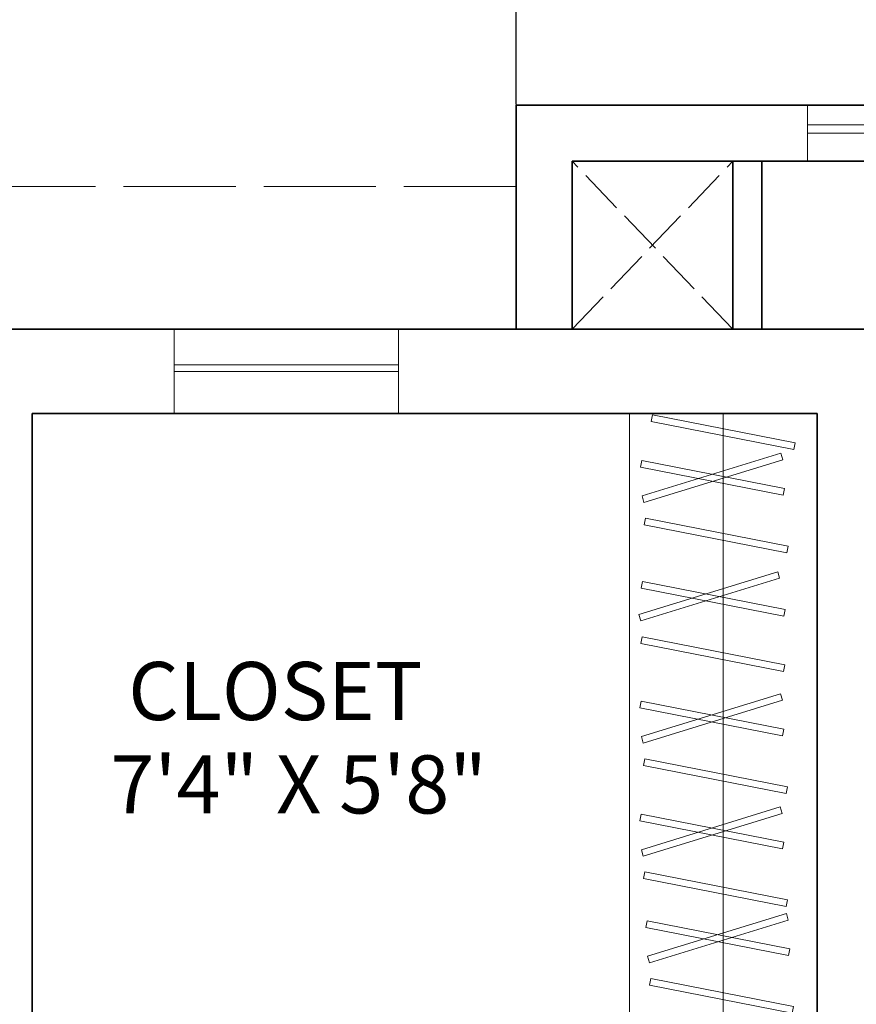
# Model space of a CAD drawing. Units: inches. Extents: x -61 to 1599, y -1316 to 257.
# Tile 172 of 204: x 1214 to 1304, y -684 to -579. Entities that reach past the tile are written whole.
import ezdxf

# ---------------------------------------------------------------- set-up
doc = ezdxf.new("R2010")
doc.units = ezdxf.units.IN
doc.header["$MEASUREMENT"] = 0
doc.linetypes.add('ACAD_ISO02W100', pattern=[15, 12, -3])
for name, color, linetype, lineweight in [('A-ANNO-DIMS', 2, 'Continuous', 18), ('A-AREA-IDEN', 1, 'Continuous', 18), ('A-FLOR-CASE', 8, 'Continuous', 18), ('A-FLOR-OPEN-HIDN', 8, 'ACAD_ISO02W100', 13), ('A-FLOR-OVHD', 203, 'ACAD_ISO02W100', 13), ('WALLS', 4, 'Continuous', 35), ('WINDOWS', 220, 'Continuous', 18)]:
    doc.layers.add(name, color=color, linetype=linetype, lineweight=lineweight)
doc.styles.get("Standard").update_dxf_attribs({"font": 'arial.ttf'})
doc.dimstyles.get("Standard").update_dxf_attribs({"dimtxt": 0.18, "dimasz": 0.18, "dimexe": 0.18, "dimexo": 0.0625, "dimgap": 0.09, "dimtad": 0, "dimtih": 1, "dimtoh": 1, "dimdec": 0, "dimzin": 0, "dimdsep": 46, "dimlunit": 3, "dimtxsty": 'Standard', "dimcen": 0.09, "dimadec": 0, "dimazin": 0, "dimtfac": 1, "dimtdec": 0, "dimtofl": 0, "dimtmove": 0, "dimatfit": 3, "dimfxl": 1, "dimtolj": 1, "dimtzin": 0, "dimarcsym": 0})

# ---------------------------------------------------------------- blocks, each defined once
blk = doc.blocks.new('WIN-24IN')
for p, q in [((0, 4.5), (0, 9)), ((0, 9), (0, 0)), ((24, 9), (24, 0)), ((0, 5.19), (24, 5.19)), ((0, 4.5), (24, 4.5))]:
    blk.add_line(p, q)
blk = doc.blocks.new('WIN-51IN')
for p, q in [((0, 0), (0, 6)), ((50.52, 0), (50.52, 6)), ((0, 3.89), (50.52, 3.89)), ((0, 3), (50.52, 3))]:
    blk.add_line(p, q)
blk = doc.blocks.new('WARDROBE-HANGING')
blk.add_line((10.05, 0), (10.05, 68))
for points in [[(20.09, 0), (0, 0), (0, 68), (20.09, 68)], [(2.48, 67.85), (17.75, 64.85), (17.61, 64.14), (2.34, 67.15)], [(1.35, 59.16), (16.22, 63.73), (16.43, 63.04), (1.56, 58.47)], [(1.32, 62.96), (16.59, 59.95), (16.45, 59.25), (1.19, 62.25)], [(1.71, 56.78), (16.98, 53.78), (16.84, 53.07), (1.57, 56.08)], [(1, 46.47), (15.87, 51.04), (16.08, 50.35), (1.21, 45.78)], [(1.39, 50.01), (16.66, 47.01), (16.52, 46.3), (1.26, 49.31)], [(1.36, 44.09), (16.63, 41.09), (16.49, 40.38), (1.23, 43.38)], [(1.28, 33.41), (16.16, 37.98), (16.37, 37.29), (1.49, 32.72)], [(1.26, 37.2), (16.53, 34.2), (16.39, 33.49), (1.12, 36.5)], [(1.65, 31.03), (16.92, 28.03), (16.78, 27.32), (1.51, 30.32)], [(1.28, 21.3), (16.15, 25.87), (16.36, 25.18), (1.49, 20.61)], [(1.26, 25.09), (16.53, 22.09), (16.39, 21.38), (1.12, 24.39)], [(1.65, 18.92), (16.91, 15.92), (16.78, 15.21), (1.51, 18.21)], [(1.93, 9.89), (16.8, 14.46), (17.01, 13.77), (2.14, 9.2)], [(1.91, 13.69), (17.17, 10.68), (17.04, 9.98), (1.77, 12.98)], [(2.29, 7.51), (17.56, 4.51), (17.42, 3.8), (2.16, 6.81)], [(17.49, 1.96), (1.93, 1.96), (1.93, 2.68), (17.49, 2.68)]]:
    blk.add_lwpolyline(points, close=True)
blk = doc.blocks.new('*D708')
at = {"layer": 'A-ANNO-DIMS', "color": 0, "lineweight": -2, "transparency": 16777216}
for p, q in [((1267.48, -588.11), (1267.48, 257.46)), ((1267.66, 257.28), (1324.14, 257.28)), ((1381.52, 257.28), (1325.05, 257.28)), ((1381.7, -588.11), (1381.7, 257.46))]:
    blk.add_line(p, q, dxfattribs=at)
at = {"layer": 'A-ANNO-DIMS', "color": 0, "transparency": 16777216}
for points in [[(1267.66, 257.31), (1267.66, 257.25), (1267.48, 257.28)], [(1381.52, 257.31), (1381.52, 257.25), (1381.7, 257.28)]]:
    blk.add_solid(points, dxfattribs=at)
at = {"layer": 'DEFPOINTS', "color": 0, "transparency": 16777216}
for p in [(1381.7, 257.28), (1267.48, -588.17), (1381.7, -588.17)]:
    blk.add_point(p, dxfattribs=at)
at = {"layer": 'A-ANNO-DIMS', "color": 0, "transparency": 16777216, "insert": (1324.59, 257.28), "char_height": 0.18, "attachment_point": 5}
blk.add_mtext('\\A1;114.22', dxfattribs=at)

msp = doc.modelspace()

# ---------------------------------------------------------------- linework, layer by layer
at = {"layer": 'A-FLOR-OPEN-HIDN', "ltscale": 0.4}
for p, q in [((1273.4807, -612.169), (1290.6819, -594.169)), ((1290.6819, -612.169), (1273.4807, -594.169))]:
    msp.add_line(p, q, dxfattribs=at)
at = {"layer": 'A-FLOR-OVHD'}
msp.add_line((1267.4807, -596.8766), (1138.8585, -596.8766), dxfattribs=at)
at = {"layer": 'WALLS'}
for p, q in [((1267.4807, -612.169), (1267.4807, -588.169)), ((1381.7028, -588.169), (1267.4807, -588.169)), ((1273.4807, -612.169), (1273.4807, -594.169)), ((1375.7028, -594.169), (1273.4807, -594.169)), ((1290.6819, -612.169), (1290.6819, -594.169)), ((1293.7747, -612.169), (1293.7747, -594.169)), ((1522.7028, -612.169), (992.7028, -612.169)), ((1215.7028, -621.169), (1215.7028, -689.169)), ((1215.7028, -621.169), (1299.7028, -621.169)), ((1299.7028, -621.169), (1299.7028, -689.169))]:
    msp.add_line(p, q, dxfattribs=at)

# ---------------------------------------------------------------- block references
at = {"layer": 'A-FLOR-CASE'}
msp.add_blockref('WARDROBE-HANGING', (1279.609, -689.1691), dxfattribs=at)
at = {"layer": 'WINDOWS'}
for name, p in [('WIN-51IN', (1298.659, -594.1691)), ('WIN-24IN', (1230.882, -621.1691))]:
    msp.add_blockref(name, p, dxfattribs=at)

# ---------------------------------------------------------------- texts
at = {"layer": 'A-AREA-IDEN'}
for s, height, p in [('   CLOSET', 6.22364, (1220.2634, -653.9959)), ('  7\'4" X 5\'8"', 6.223643, (1220.2634, -663.9936))]:
    msp.add_text(s, height=height, dxfattribs=at).set_placement(p)

# ---------------------------------------------------------------- dimensions: what is measured, and where the dimension line sits
at = {"layer": 'A-ANNO-DIMS'}
dim = msp.add_linear_dim(base=(1381.7028, 257.2771), p1=(1267.4807, -588.169), p2=(1381.7028, -588.169), dimstyle='Standard', override={"dimdec": 2, "dimlfac": 1, "dimrnd": 0, "dimzin": 0, "dimdsep": 46, "dimlunit": 2}, dxfattribs=at)
dim.commit()
dim.dimension.update_dxf_attribs({"geometry": '*D708', "text_midpoint": (1324.5917, 257.2771)})

doc.saveas('drawing.dxf')
